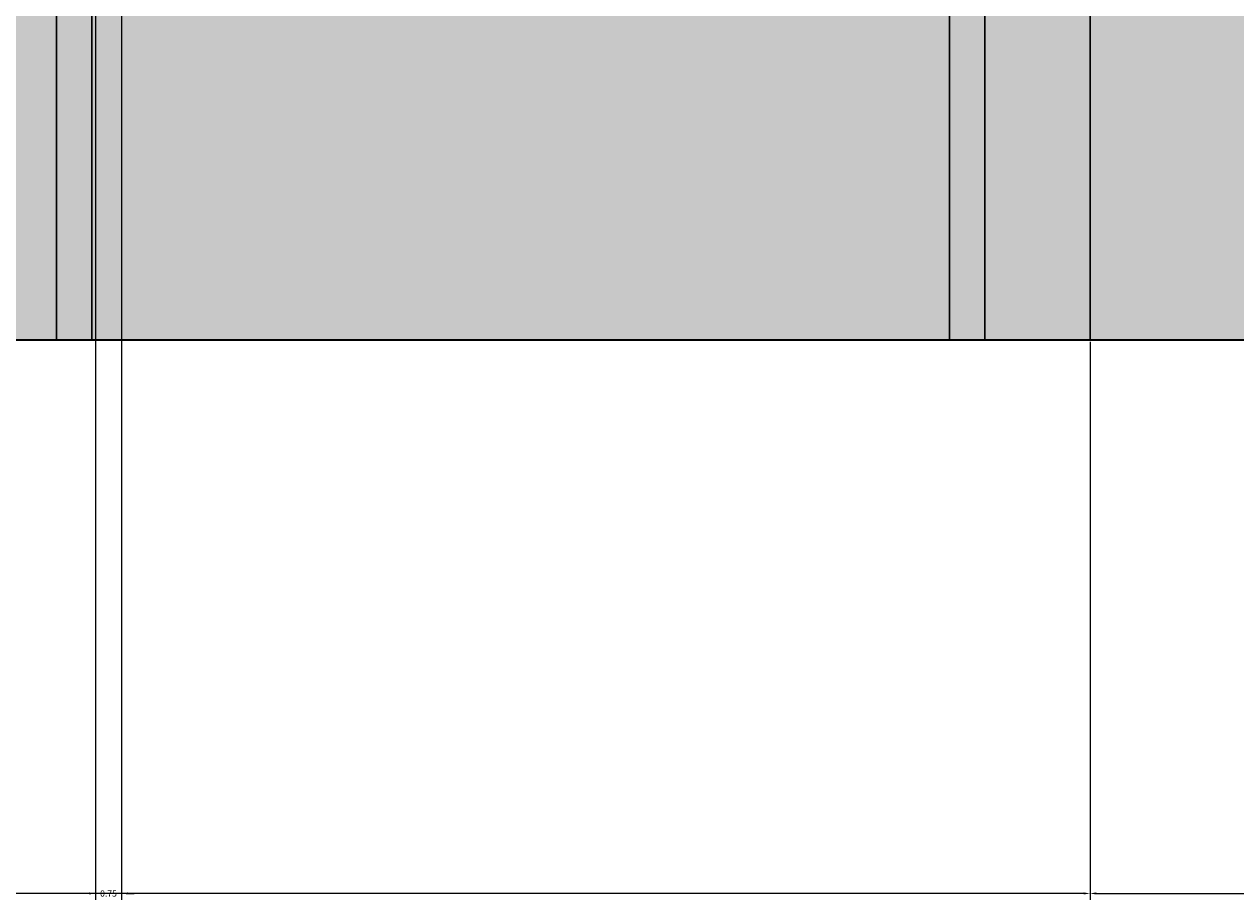
# Model space of a CAD drawing. Units: feet. Extents: x 2695 to 2912, y 795 to 1139.
# Tile 18 of 83: x 2808 to 2843, y 795 to 820. Entities that reach past the tile are written whole.
import ezdxf

# ---------------------------------------------------------------- set-up
doc = ezdxf.new("R2010")
doc.units = ezdxf.units.FT
for name, color, linetype, lineweight in [('A-ANNO-DIMS', 2, 'Continuous', 18), ('A-DOOR', 3, 'Continuous', 25), ('A-DOOR-PATT', 33, 'Continuous', 13), ('A-ELEV', 7, 'Continuous', 35), ('A-ELEV-PATT', 252, 'Continuous', 13)]:
    doc.layers.add(name, color=color, linetype=linetype, lineweight=lineweight)
doc.styles.get("Standard").update_dxf_attribs({"font": 'arial.ttf'})
doc.dimstyles.get("Standard").update_dxf_attribs({"dimtxt": 0.18, "dimasz": 0.18, "dimexe": 0.18, "dimexo": 0.0625, "dimgap": 0.09, "dimtad": 0, "dimtih": 1, "dimtoh": 1, "dimdec": 1, "dimzin": 0, "dimdsep": 46, "dimlunit": 3, "dimtxsty": 'Standard', "dimcen": 0.09, "dimadec": 0, "dimazin": 0, "dimtfac": 1, "dimtdec": 1, "dimtofl": 0, "dimtmove": 0, "dimatfit": 3, "dimfxl": 1, "dimtolj": 1, "dimtzin": 0, "dimarcsym": 0})

# ---------------------------------------------------------------- blocks, each defined once
blk = doc.blocks.new('*D5')
at = {"layer": 'A-ANNO-DIMS', "color": 0, "lineweight": -2, "transparency": 16777216}
for p, q in [((2773.503, 810.868), (2773.503, 794.976)), ((2838.377, 810.868), (2838.377, 794.976)), ((2773.683, 795.156), (2805.546, 795.156)), ((2838.197, 795.156), (2806.334, 795.156))]:
    blk.add_line(p, q, dxfattribs=at)
at = {"layer": 'A-ANNO-DIMS', "color": 0, "transparency": 16777216}
for points in [[(2773.683, 795.186), (2773.683, 795.126), (2773.503, 795.156)], [(2838.197, 795.186), (2838.197, 795.126), (2838.377, 795.156)]]:
    blk.add_solid(points, dxfattribs=at)
at = {"layer": 'Defpoints', "color": 0, "transparency": 16777216}
for p in [(2773.503, 810.931), (2838.377, 810.931), (2838.377, 795.156)]:
    blk.add_point(p, dxfattribs=at)
at = {"layer": 'A-ANNO-DIMS', "color": 0, "transparency": 16777216, "insert": (2805.94, 795.156), "char_height": 0.18, "attachment_point": 5}
blk.add_mtext('\\A1;64.87', dxfattribs=at)
blk = doc.blocks.new('*D6')
at = {"layer": 'A-ANNO-DIMS', "color": 0, "lineweight": -2, "transparency": 16777216}
for p, q in [((2838.377, 810.868), (2838.377, 794.976)), ((2890.636, 810.868), (2890.636, 794.976)), ((2838.557, 795.156), (2864.113, 795.156)), ((2890.456, 795.156), (2864.9, 795.156))]:
    blk.add_line(p, q, dxfattribs=at)
at = {"layer": 'A-ANNO-DIMS', "color": 0, "transparency": 16777216}
for points in [[(2838.557, 795.186), (2838.557, 795.126), (2838.377, 795.156)], [(2890.456, 795.186), (2890.456, 795.126), (2890.636, 795.156)]]:
    blk.add_solid(points, dxfattribs=at)
at = {"layer": 'Defpoints', "color": 0, "transparency": 16777216}
for p in [(2838.377, 810.931), (2890.636, 810.931), (2890.636, 795.156)]:
    blk.add_point(p, dxfattribs=at)
at = {"layer": 'A-ANNO-DIMS', "color": 0, "transparency": 16777216, "insert": (2864.506, 795.156), "char_height": 0.18, "attachment_point": 5}
blk.add_mtext('\\A1;52.26', dxfattribs=at)
blk = doc.blocks.new('*D13')
at = {"layer": 'A-ANNO-DIMS', "color": 0, "lineweight": -2, "transparency": 16777216}
for p, q in [((2758.214, 874.857), (2911.424, 874.857)), ((2911.244, 874.677), (2911.244, 843.076)), ((2911.244, 811.111), (2911.244, 842.712)), ((2890.699, 810.931), (2911.424, 810.931))]:
    blk.add_line(p, q, dxfattribs=at)
at = {"layer": 'A-ANNO-DIMS', "color": 0, "transparency": 16777216}
for points in [[(2911.214, 874.677), (2911.274, 874.677), (2911.244, 874.857)], [(2911.214, 811.111), (2911.274, 811.111), (2911.244, 810.931)]]:
    blk.add_solid(points, dxfattribs=at)
at = {"layer": 'Defpoints', "color": 0, "transparency": 16777216}
for p in [(2758.151, 874.857), (2911.244, 874.857), (2890.636, 810.931)]:
    blk.add_point(p, dxfattribs=at)
at = {"layer": 'A-ANNO-DIMS', "color": 0, "transparency": 16777216, "insert": (2911.244, 842.894), "char_height": 0.18, "attachment_point": 5}
blk.add_mtext('\\A1;63.93', dxfattribs=at)
blk = doc.blocks.new('*D52')
at = {"layer": 'A-ANNO-DIMS', "color": 0, "lineweight": -2, "transparency": 16777216}
for p, q in [((2810.041, 936.868), (2810.041, 794.976)), ((2810.789, 936.868), (2810.789, 794.976)), ((2809.861, 795.156), (2809.681, 795.156)), ((2810.969, 795.156), (2811.149, 795.156))]:
    blk.add_line(p, q, dxfattribs=at)
at = {"layer": 'A-ANNO-DIMS', "color": 0, "transparency": 16777216}
for points in [[(2809.861, 795.186), (2809.861, 795.126), (2810.041, 795.156)], [(2810.969, 795.186), (2810.969, 795.126), (2810.789, 795.156)]]:
    blk.add_solid(points, dxfattribs=at)
at = {"layer": 'Defpoints', "color": 0, "transparency": 16777216}
for p in [(2810.041, 936.931), (2810.789, 936.931), (2810.789, 795.156)]:
    blk.add_point(p, dxfattribs=at)
at = {"layer": 'A-ANNO-DIMS', "color": 0, "transparency": 16777216, "insert": (2810.415, 795.156), "char_height": 0.18, "attachment_point": 5}
blk.add_mtext('\\A1;0.75', dxfattribs=at)

msp = doc.modelspace()

# ---------------------------------------------------------------- hatches: boundary and pattern name
at = {"layer": 'A-DOOR-PATT'}
h = msp.add_hatch(color=256, dxfattribs=at)
h.set_gradient(color1=(211, 185, 150), color2=(211, 185, 150))
h.paths.add_polyline_path([(2805.9398, 905.5143), (2773.5029, 905.5143), (2773.5029, 810.9306), (2776.4999, 810.9306), (2776.4999, 902.5174), (2802.9429, 902.5174), (2802.9429, 810.9306), (2805.9398, 810.9306)])
h.paths.add_polyline_path([(2803.9681, 874.1057), (2805.0538, 874.1057), (2805.0538, 846.2857), (2803.9681, 846.2857)], flags=16)
h.paths.add_polyline_path([(2838.3767, 905.5143), (2805.9398, 905.5143), (2805.9398, 810.9306), (2808.9368, 810.9306), (2808.9368, 902.5174), (2835.3798, 902.5174), (2835.3798, 810.9306), (2838.3767, 810.9306)])
h = msp.add_hatch(color=256, dxfattribs=at)
h.set_gradient(color1=(211, 185, 150), color2=(211, 185, 150))
h.paths.add_polyline_path([(2777.5029, 901.5143), (2801.9398, 901.5143), (2801.9398, 810.9306), (2802.9429, 810.9306), (2802.9429, 902.5174), (2776.4999, 902.5174), (2776.4999, 810.9306), (2777.5029, 810.9306)])
h.paths.add_polyline_path([(2809.9398, 901.5143), (2834.3767, 901.5143), (2834.3767, 810.9306), (2835.3798, 810.9306), (2835.3798, 902.5174), (2808.9368, 902.5174), (2808.9368, 810.9306), (2809.9398, 810.9306)])
h = msp.add_hatch(color=256, dxfattribs=at)
h.set_gradient(color1=(173, 221, 247), color2=(173, 221, 247))
h.paths.add_polyline_path([(2801.9398, 901.5143), (2777.5029, 901.5143), (2777.5029, 810.9306), (2801.9398, 810.9306)])
h.paths.add_polyline_path([(2834.3767, 901.5143), (2809.9398, 901.5143), (2809.9398, 810.9306), (2834.3767, 810.9306)])
at = {"layer": 'A-ELEV-PATT'}
h = msp.add_hatch(color=256, dxfattribs=at)
h.set_gradient(color1=(147, 149, 152), color2=(147, 149, 152), tint=1)
h.paths.add_polyline_path([(2770.6361, 1118.4096), (2710.6361, 1118.4096), (2710.6361, 1062.9306), (2770.6361, 1062.9306)])
h.paths.add_polyline_path([(2890.6361, 1103.3378), (2770.6361, 1103.3378), (2770.6361, 1062.9306), (2890.6361, 1062.9306)])
h.paths.add_polyline_path([(2730.7081, 1048.1052), (2755.1125, 1048.1052), (2755.1125, 936.9306), (2770.6361, 936.9306), (2770.6361, 1050.3105), (2715.8852, 1050.3105), (2715.8852, 936.9306), (2730.7081, 936.9306)])
h.paths.add_polyline_path([(2890.6361, 1050.3105), (2770.6361, 1050.3105), (2770.6361, 971.9673), (2778.0341, 971.9673), (2778.0341, 1020.8235), (2843.575, 1020.8235), (2843.575, 971.9673), (2890.6361, 971.9673)])
h.paths.add_polyline_path([(2888.1882, 970.7156), (2843.575, 970.7156), (2843.575, 964.8267), (2888.1882, 964.8267)])
h.paths.add_polyline_path([(2888.1882, 964.1328), (2843.575, 964.1328), (2843.575, 956.614), (2888.1882, 956.614)])
h.paths.add_polyline_path([(2888.1882, 955.9202), (2843.575, 955.9202), (2843.575, 949.2892), (2888.1882, 949.2892)])
h.paths.add_polyline_path([(2888.1882, 948.5954), (2843.575, 948.5954), (2843.575, 941.3507), (2888.1882, 941.3507)])
h.paths.add_polyline_path([(2888.1882, 940.6569), (2843.575, 940.6569), (2843.575, 936.9306), (2888.1882, 936.9306)])
h.paths.add_polyline_path([(2890.6361, 970.7156), (2888.9368, 970.7156), (2888.9368, 964.8267), (2890.6361, 964.8267)])
h.paths.add_polyline_path([(2890.6361, 964.1328), (2888.9368, 964.1328), (2888.9368, 956.614), (2890.6361, 956.614)])
h.paths.add_polyline_path([(2890.6361, 955.9202), (2888.9368, 955.9202), (2888.9368, 949.2892), (2890.6361, 949.2892)])
h.paths.add_polyline_path([(2890.6361, 940.6569), (2888.9368, 940.6569), (2888.9368, 936.9306), (2890.6361, 936.9306)])
h.paths.add_polyline_path([(2890.6361, 948.5954), (2888.9368, 948.5954), (2888.9368, 941.3507), (2890.6361, 941.3507)])
h.paths.add_polyline_path([(2772.5216, 970.7156), (2770.6361, 970.7156), (2770.6361, 964.8267), (2772.5216, 964.8267)])
h.paths.add_polyline_path([(2772.5216, 964.1328), (2770.6361, 964.1328), (2770.6361, 956.614), (2772.5216, 956.614)])
h.paths.add_polyline_path([(2772.5216, 955.9202), (2770.6361, 955.9202), (2770.6361, 949.2892), (2772.5216, 949.2892)])
h.paths.add_polyline_path([(2772.5216, 948.5954), (2770.6361, 948.5954), (2770.6361, 941.3507), (2772.5216, 941.3507)])
h.paths.add_polyline_path([(2772.5216, 940.6569), (2770.6361, 940.6569), (2770.6361, 936.9306), (2772.5216, 936.9306)])
h.paths.add_polyline_path([(2778.0341, 940.6569), (2773.2702, 940.6569), (2773.2702, 936.9306), (2778.0341, 936.9306)])
h.paths.add_polyline_path([(2778.0341, 970.7156), (2773.2702, 970.7156), (2773.2702, 964.8267), (2778.0341, 964.8267)])
h.paths.add_polyline_path([(2778.0341, 964.1328), (2773.2702, 964.1328), (2773.2702, 956.614), (2778.0341, 956.614)])
h.paths.add_polyline_path([(2778.0341, 955.9202), (2773.2702, 955.9202), (2773.2702, 949.2892), (2778.0341, 949.2892)])
h.paths.add_polyline_path([(2778.0341, 948.5954), (2773.2702, 948.5954), (2773.2702, 941.3507), (2778.0341, 941.3507)])
h.paths.add_polyline_path([(2810.0407, 940.6569), (2780.0341, 940.6569), (2780.0341, 936.9306), (2810.0407, 936.9306)])
h.paths.add_polyline_path([(2890.6361, 924.3105), (2770.6361, 924.3105), (2770.6361, 810.9306), (2773.5029, 810.9306), (2773.5029, 905.5143), (2805.9398, 905.5143), (2838.3767, 905.5143), (2838.3767, 810.9306), (2890.6361, 810.9306)])

# ---------------------------------------------------------------- linework, layer by layer
at = {"layer": 'A-DOOR'}
for points in [[(2773.5029, 905.5143), (2838.3767, 905.5143), (2838.3767, 810.9306), (2773.5029, 810.9306)], [(2808.9368, 902.5174), (2835.3798, 902.5174), (2835.3798, 810.9306), (2808.9368, 810.9306)], [(2809.9398, 901.5143), (2834.3767, 901.5143), (2834.3767, 810.9306), (2809.9398, 810.9306)]]:
    msp.add_lwpolyline(points, close=True, dxfattribs=at)
for points in [[(2838.3767, 810.9306), (2838.3767, 905.5143), (2805.9398, 905.5143), (2805.9398, 810.9306)], [(2835.3798, 810.9306), (2835.3798, 902.5174), (2808.9368, 902.5174), (2808.9368, 810.9306)], [(2834.3767, 810.9306), (2834.3767, 901.5143), (2809.9398, 901.5143), (2809.9398, 810.9306)]]:
    msp.add_lwpolyline(points, dxfattribs=at)
at = {"layer": 'A-ELEV'}
for q in [(2890.6361, 810.9306), (2890.6361, 810.9306), (2895.4426, 810.9306)]:
    msp.add_line((2710.6361, 810.9306), q, dxfattribs=at)

# ---------------------------------------------------------------- dimensions: what is measured, and where the dimension line sits
at = {"layer": 'A-ANNO-DIMS'}
for base, p1, p2, picture, middle in [((2810.7893, 795.1556), (2810.0407, 936.9306), (2810.7893, 936.9306), '*D52', (2810.415, 795.1556)), ((2838.3767, 795.1556), (2773.5029, 810.9306), (2838.3767, 810.9306), '*D5', (2805.9398, 795.1556)), ((2890.6361, 795.1556), (2838.3767, 810.9306), (2890.6361, 810.9306), '*D6', (2864.5064, 795.1556))]:
    dim = msp.add_linear_dim(base=base, p1=p1, p2=p2, dimstyle='Standard', override={"dimdec": 2, "dimlfac": 1, "dimrnd": 0, "dimzin": 0, "dimdsep": 46, "dimlunit": 2}, dxfattribs=at)
    dim.commit()
    dim.dimension.update_dxf_attribs({"geometry": picture, "text_midpoint": middle})
dim = msp.add_linear_dim(base=(2911.2444, 874.8571), p1=(2890.6361, 810.9306), p2=(2758.1515, 874.8571), angle=90, dimstyle='Standard', override={"dimdec": 2, "dimlfac": 1, "dimrnd": 0, "dimzin": 0, "dimdsep": 46, "dimlunit": 2}, dxfattribs=at)
dim.commit()
dim.dimension.update_dxf_attribs({"geometry": '*D13', "text_midpoint": (2911.2444, 842.8938)})

doc.saveas('drawing.dxf')
